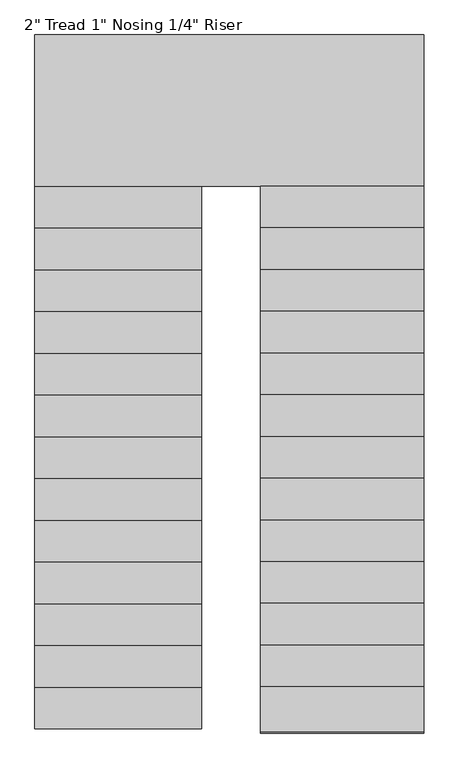
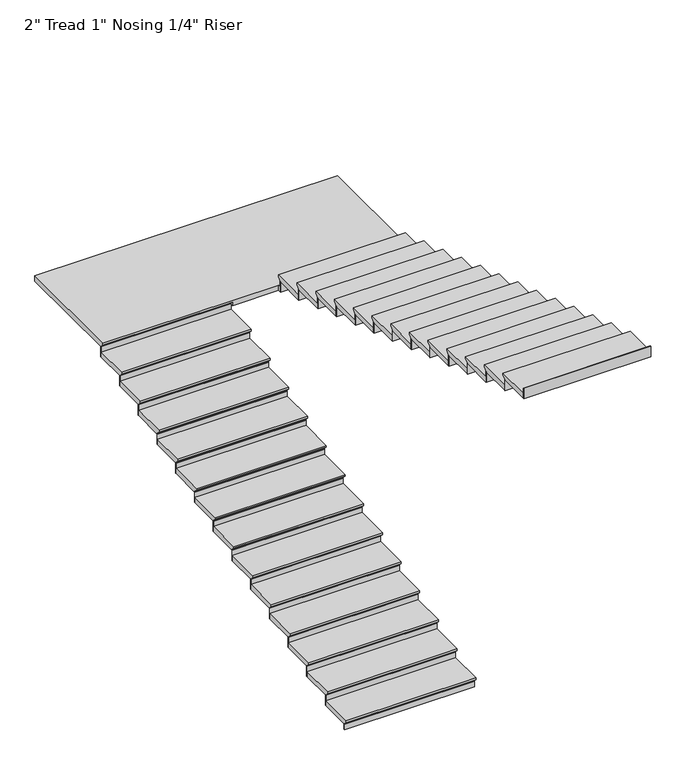
"""IFC4 building model written with IfcOpenShell, lengths in millimetres: stair flight geometry."""

from ifc_helpers import new_model, si_unit, origin, place, context, project, spatial, faceted_brep, source, transform, mapped, element, save


def stair_flight_d8047cd6(model_context):
    return source(origin(), model_context, "Body", "Brep", [
        faceted_brep([(-629.5987998, 2564.5067329, 16086.3642857), (-629.5987998, 2564.5067329, 16105.4142857), (-1848.7987998, 2564.5067329, 16105.4142857), (-1848.7987998, 2564.5067329, 16086.3642857), (-629.5987998, 2589.9067329, 16060.9642857), (-1848.7987998, 2589.9067329, 16060.9642857), (-629.5987998, 2894.7067329, 16105.4142857), (-1848.7987998, 2894.7067329, 16105.4142857), (-1848.7987998, 2589.9067329, 16054.6142857), (-1848.7987998, 2894.7067329, 16054.6142857), (-629.5987998, 2894.7067329, 16054.6142857), (-629.5987998, 2589.9067329, 16054.6142857)], [[[0, 1, 2, 3]], [[4, 0, 3, 5]], [[2, 1, 6, 7]], [[8, 9, 10, 11]], [[2, 7, 9, 8, 5, 3]], [[8, 11, 4, 5]], [[6, 1, 0, 4, 11, 10]], [[7, 6, 10, 9]]]),
        faceted_brep([(-629.5987998, 2589.9067329, 16054.6142857), (-629.5987998, 2589.9067329, 16002.0), (-629.5987998, 2596.2567329, 16002.0), (-629.5987998, 2596.2567329, 16054.6142857), (-1848.7987998, 2589.9067329, 16054.6142857), (-1848.7987998, 2596.2567329, 16054.6142857), (-1848.7987998, 2596.2567329, 16002.0), (-1848.7987998, 2589.9067329, 16002.0)], [[[0, 1, 2, 3]], [[4, 5, 6, 7]], [[1, 0, 4, 7]], [[2, 1, 7, 6]], [[3, 2, 6, 5]], [[0, 3, 5, 4]]]),
        faceted_brep([(-629.5987998, 2894.7067329, 16158.0285714), (-629.5987998, 2894.7067329, 16054.6142857), (-629.5987998, 2901.0567329, 16054.6142857), (-629.5987998, 2901.0567329, 16158.0285714), (-1848.7987998, 2894.7067329, 16158.0285714), (-1848.7987998, 2901.0567329, 16158.0285714), (-1848.7987998, 2901.0567329, 16054.6142857), (-1848.7987998, 2894.7067329, 16054.6142857)], [[[0, 1, 2, 3]], [[4, 5, 6, 7]], [[1, 0, 4, 7]], [[2, 1, 7, 6]], [[3, 2, 6, 5]], [[0, 3, 5, 4]]]),
        faceted_brep([(-1848.7987998, 2869.3067329, 16208.8285714), (-629.5987998, 2869.3067329, 16208.8285714), (-629.5987998, 3199.5067329, 16208.8285714), (-1848.7987998, 3199.5067329, 16208.8285714), (-1848.7987998, 2894.7067329, 16158.0285714), (-1848.7987998, 3199.5067329, 16158.0285714), (-629.5987998, 3199.5067329, 16158.0285714), (-629.5987998, 2894.7067329, 16158.0285714), (-1848.7987998, 2894.7067329, 16164.3785714), (-1848.7987998, 2869.3067329, 16189.7785714), (-629.5987998, 2894.7067329, 16164.3785714), (-629.5987998, 2869.3067329, 16189.7785714)], [[[0, 1, 2, 3]], [[4, 5, 6, 7]], [[0, 3, 5, 4, 8, 9]], [[4, 7, 10, 8]], [[2, 1, 11, 10, 7, 6]], [[3, 2, 6, 5]], [[11, 1, 0, 9]], [[10, 11, 9, 8]]]),
        faceted_brep([(-629.5987998, 3199.5067329, 16261.4428571), (-629.5987998, 3199.5067329, 16158.0285714), (-629.5987998, 3205.8567329, 16158.0285714), (-629.5987998, 3205.8567329, 16261.4428571), (-1848.7987998, 3199.5067329, 16261.4428571), (-1848.7987998, 3205.8567329, 16261.4428571), (-1848.7987998, 3205.8567329, 16158.0285714), (-1848.7987998, 3199.5067329, 16158.0285714)], [[[0, 1, 2, 3]], [[4, 5, 6, 7]], [[1, 0, 4, 7]], [[2, 1, 7, 6]], [[3, 2, 6, 5]], [[0, 3, 5, 4]]]),
        faceted_brep([(-1848.7987998, 3174.1067329, 16312.2428571), (-629.5987998, 3174.1067329, 16312.2428571), (-629.5987998, 3504.3067329, 16312.2428571), (-1848.7987998, 3504.3067329, 16312.2428571), (-1848.7987998, 3199.5067329, 16261.4428571), (-1848.7987998, 3504.3067329, 16261.4428571), (-629.5987998, 3504.3067329, 16261.4428571), (-629.5987998, 3199.5067329, 16261.4428571), (-1848.7987998, 3199.5067329, 16267.7928571), (-1848.7987998, 3174.1067329, 16293.1928571), (-629.5987998, 3199.5067329, 16267.7928571), (-629.5987998, 3174.1067329, 16293.1928571)], [[[0, 1, 2, 3]], [[4, 5, 6, 7]], [[0, 3, 5, 4, 8, 9]], [[4, 7, 10, 8]], [[2, 1, 11, 10, 7, 6]], [[3, 2, 6, 5]], [[11, 1, 0, 9]], [[10, 11, 9, 8]]]),
        faceted_brep([(-629.5987998, 3504.3067329, 16364.8571429), (-629.5987998, 3504.3067329, 16261.4428571), (-629.5987998, 3510.6567329, 16261.4428571), (-629.5987998, 3510.6567329, 16364.8571429), (-1848.7987998, 3504.3067329, 16364.8571429), (-1848.7987998, 3510.6567329, 16364.8571429), (-1848.7987998, 3510.6567329, 16261.4428571), (-1848.7987998, 3504.3067329, 16261.4428571)], [[[0, 1, 2, 3]], [[4, 5, 6, 7]], [[1, 0, 4, 7]], [[2, 1, 7, 6]], [[3, 2, 6, 5]], [[0, 3, 5, 4]]]),
        faceted_brep([(-1848.7987998, 3478.9067329, 16415.6571429), (-629.5987998, 3478.9067329, 16415.6571429), (-629.5987998, 3809.1067329, 16415.6571429), (-1848.7987998, 3809.1067329, 16415.6571429), (-1848.7987998, 3504.3067329, 16364.8571429), (-1848.7987998, 3809.1067329, 16364.8571429), (-629.5987998, 3809.1067329, 16364.8571429), (-629.5987998, 3504.3067329, 16364.8571429), (-1848.7987998, 3504.3067329, 16371.2071429), (-1848.7987998, 3478.9067329, 16396.6071429), (-629.5987998, 3504.3067329, 16371.2071429), (-629.5987998, 3478.9067329, 16396.6071429)], [[[0, 1, 2, 3]], [[4, 5, 6, 7]], [[0, 3, 5, 4, 8, 9]], [[4, 7, 10, 8]], [[2, 1, 11, 10, 7, 6]], [[3, 2, 6, 5]], [[11, 1, 0, 9]], [[10, 11, 9, 8]]]),
        faceted_brep([(-629.5987998, 3809.1067329, 16468.2714286), (-629.5987998, 3809.1067329, 16364.8571429), (-629.5987998, 3815.4567329, 16364.8571429), (-629.5987998, 3815.4567329, 16468.2714286), (-1848.7987998, 3809.1067329, 16468.2714286), (-1848.7987998, 3815.4567329, 16468.2714286), (-1848.7987998, 3815.4567329, 16364.8571429), (-1848.7987998, 3809.1067329, 16364.8571429)], [[[0, 1, 2, 3]], [[4, 5, 6, 7]], [[1, 0, 4, 7]], [[2, 1, 7, 6]], [[3, 2, 6, 5]], [[0, 3, 5, 4]]]),
        faceted_brep([(-1848.7987998, 3783.7067329, 16519.0714286), (-629.5987998, 3783.7067329, 16519.0714286), (-629.5987998, 4113.9067329, 16519.0714286), (-1848.7987998, 4113.9067329, 16519.0714286), (-1848.7987998, 3809.1067329, 16468.2714286), (-1848.7987998, 4113.9067329, 16468.2714286), (-629.5987998, 4113.9067329, 16468.2714286), (-629.5987998, 3809.1067329, 16468.2714286), (-1848.7987998, 3809.1067329, 16474.6214286), (-1848.7987998, 3783.7067329, 16500.0214286), (-629.5987998, 3809.1067329, 16474.6214286), (-629.5987998, 3783.7067329, 16500.0214286)], [[[0, 1, 2, 3]], [[4, 5, 6, 7]], [[0, 3, 5, 4, 8, 9]], [[4, 7, 10, 8]], [[2, 1, 11, 10, 7, 6]], [[3, 2, 6, 5]], [[11, 1, 0, 9]], [[10, 11, 9, 8]]]),
        faceted_brep([(-629.5987998, 4113.9067329, 16571.6857143), (-629.5987998, 4113.9067329, 16468.2714286), (-629.5987998, 4120.2567329, 16468.2714286), (-629.5987998, 4120.2567329, 16571.6857143), (-1848.7987998, 4113.9067329, 16571.6857143), (-1848.7987998, 4120.2567329, 16571.6857143), (-1848.7987998, 4120.2567329, 16468.2714286), (-1848.7987998, 4113.9067329, 16468.2714286)], [[[0, 1, 2, 3]], [[4, 5, 6, 7]], [[1, 0, 4, 7]], [[2, 1, 7, 6]], [[3, 2, 6, 5]], [[0, 3, 5, 4]]]),
        faceted_brep([(-1848.7987998, 4088.5067329, 16622.4857143), (-629.5987998, 4088.5067329, 16622.4857143), (-629.5987998, 4418.7067329, 16622.4857143), (-1848.7987998, 4418.7067329, 16622.4857143), (-1848.7987998, 4113.9067329, 16571.6857143), (-1848.7987998, 4418.7067329, 16571.6857143), (-629.5987998, 4418.7067329, 16571.6857143), (-629.5987998, 4113.9067329, 16571.6857143), (-1848.7987998, 4113.9067329, 16578.0357143), (-1848.7987998, 4088.5067329, 16603.4357143), (-629.5987998, 4113.9067329, 16578.0357143), (-629.5987998, 4088.5067329, 16603.4357143)], [[[0, 1, 2, 3]], [[4, 5, 6, 7]], [[0, 3, 5, 4, 8, 9]], [[4, 7, 10, 8]], [[2, 1, 11, 10, 7, 6]], [[3, 2, 6, 5]], [[11, 1, 0, 9]], [[10, 11, 9, 8]]]),
        faceted_brep([(-629.5987998, 4418.7067329, 16675.1), (-629.5987998, 4418.7067329, 16571.6857143), (-629.5987998, 4425.0567329, 16571.6857143), (-629.5987998, 4425.0567329, 16675.1), (-1848.7987998, 4418.7067329, 16675.1), (-1848.7987998, 4425.0567329, 16675.1), (-1848.7987998, 4425.0567329, 16571.6857143), (-1848.7987998, 4418.7067329, 16571.6857143)], [[[0, 1, 2, 3]], [[4, 5, 6, 7]], [[1, 0, 4, 7]], [[2, 1, 7, 6]], [[3, 2, 6, 5]], [[0, 3, 5, 4]]]),
        faceted_brep([(-1848.7987998, 4393.3067329, 16725.9), (-629.5987998, 4393.3067329, 16725.9), (-629.5987998, 4723.5067329, 16725.9), (-1848.7987998, 4723.5067329, 16725.9), (-1848.7987998, 4418.7067329, 16675.1), (-1848.7987998, 4723.5067329, 16675.1), (-629.5987998, 4723.5067329, 16675.1), (-629.5987998, 4418.7067329, 16675.1), (-1848.7987998, 4418.7067329, 16681.45), (-1848.7987998, 4393.3067329, 16706.85), (-629.5987998, 4418.7067329, 16681.45), (-629.5987998, 4393.3067329, 16706.85)], [[[0, 1, 2, 3]], [[4, 5, 6, 7]], [[0, 3, 5, 4, 8, 9]], [[4, 7, 10, 8]], [[2, 1, 11, 10, 7, 6]], [[3, 2, 6, 5]], [[11, 1, 0, 9]], [[10, 11, 9, 8]]]),
        faceted_brep([(-629.5987998, 4723.5067329, 16778.5142857), (-629.5987998, 4723.5067329, 16675.1), (-629.5987998, 4729.8567329, 16675.1), (-629.5987998, 4729.8567329, 16778.5142857), (-1848.7987998, 4723.5067329, 16778.5142857), (-1848.7987998, 4729.8567329, 16778.5142857), (-1848.7987998, 4729.8567329, 16675.1), (-1848.7987998, 4723.5067329, 16675.1)], [[[0, 1, 2, 3]], [[4, 5, 6, 7]], [[1, 0, 4, 7]], [[2, 1, 7, 6]], [[3, 2, 6, 5]], [[0, 3, 5, 4]]]),
        faceted_brep([(-1848.7987998, 4698.1067329, 16829.3142857), (-629.5987998, 4698.1067329, 16829.3142857), (-629.5987998, 5028.3067329, 16829.3142857), (-1848.7987998, 5028.3067329, 16829.3142857), (-1848.7987998, 4723.5067329, 16778.5142857), (-1848.7987998, 5028.3067329, 16778.5142857), (-629.5987998, 5028.3067329, 16778.5142857), (-629.5987998, 4723.5067329, 16778.5142857), (-1848.7987998, 4723.5067329, 16784.8642857), (-1848.7987998, 4698.1067329, 16810.2642857), (-629.5987998, 4723.5067329, 16784.8642857), (-629.5987998, 4698.1067329, 16810.2642857)], [[[0, 1, 2, 3]], [[4, 5, 6, 7]], [[0, 3, 5, 4, 8, 9]], [[4, 7, 10, 8]], [[2, 1, 11, 10, 7, 6]], [[3, 2, 6, 5]], [[11, 1, 0, 9]], [[10, 11, 9, 8]]]),
        faceted_brep([(-629.5987998, 5028.3067329, 16881.9285714), (-629.5987998, 5028.3067329, 16778.5142857), (-629.5987998, 5034.6567329, 16778.5142857), (-629.5987998, 5034.6567329, 16881.9285714), (-1848.7987998, 5028.3067329, 16881.9285714), (-1848.7987998, 5034.6567329, 16881.9285714), (-1848.7987998, 5034.6567329, 16778.5142857), (-1848.7987998, 5028.3067329, 16778.5142857)], [[[0, 1, 2, 3]], [[4, 5, 6, 7]], [[1, 0, 4, 7]], [[2, 1, 7, 6]], [[3, 2, 6, 5]], [[0, 3, 5, 4]]]),
        faceted_brep([(-1848.7987998, 5002.9067329, 16932.7285714), (-629.5987998, 5002.9067329, 16932.7285714), (-629.5987998, 5333.1067329, 16932.7285714), (-1848.7987998, 5333.1067329, 16932.7285714), (-1848.7987998, 5028.3067329, 16881.9285714), (-1848.7987998, 5333.1067329, 16881.9285714), (-629.5987998, 5333.1067329, 16881.9285714), (-629.5987998, 5028.3067329, 16881.9285714), (-1848.7987998, 5028.3067329, 16888.2785714), (-1848.7987998, 5002.9067329, 16913.6785714), (-629.5987998, 5028.3067329, 16888.2785714), (-629.5987998, 5002.9067329, 16913.6785714)], [[[0, 1, 2, 3]], [[4, 5, 6, 7]], [[0, 3, 5, 4, 8, 9]], [[4, 7, 10, 8]], [[2, 1, 11, 10, 7, 6]], [[3, 2, 6, 5]], [[11, 1, 0, 9]], [[10, 11, 9, 8]]]),
        faceted_brep([(-629.5987998, 5333.1067329, 16985.3428571), (-629.5987998, 5333.1067329, 16881.9285714), (-629.5987998, 5339.4567329, 16881.9285714), (-629.5987998, 5339.4567329, 16985.3428571), (-1848.7987998, 5333.1067329, 16985.3428571), (-1848.7987998, 5339.4567329, 16985.3428571), (-1848.7987998, 5339.4567329, 16881.9285714), (-1848.7987998, 5333.1067329, 16881.9285714)], [[[0, 1, 2, 3]], [[4, 5, 6, 7]], [[1, 0, 4, 7]], [[2, 1, 7, 6]], [[3, 2, 6, 5]], [[0, 3, 5, 4]]]),
        faceted_brep([(-1848.7987998, 5307.7067329, 17036.1428571), (-629.5987998, 5307.7067329, 17036.1428571), (-629.5987998, 5637.9067329, 17036.1428571), (-1848.7987998, 5637.9067329, 17036.1428571), (-1848.7987998, 5333.1067329, 16985.3428571), (-1848.7987998, 5637.9067329, 16985.3428571), (-629.5987998, 5637.9067329, 16985.3428571), (-629.5987998, 5333.1067329, 16985.3428571), (-1848.7987998, 5333.1067329, 16991.6928571), (-1848.7987998, 5307.7067329, 17017.0928571), (-629.5987998, 5333.1067329, 16991.6928571), (-629.5987998, 5307.7067329, 17017.0928571)], [[[0, 1, 2, 3]], [[4, 5, 6, 7]], [[0, 3, 5, 4, 8, 9]], [[4, 7, 10, 8]], [[2, 1, 11, 10, 7, 6]], [[3, 2, 6, 5]], [[11, 1, 0, 9]], [[10, 11, 9, 8]]]),
        faceted_brep([(-629.5987998, 5637.9067329, 17088.7571429), (-629.5987998, 5637.9067329, 16985.3428571), (-629.5987998, 5644.2567329, 16985.3428571), (-629.5987998, 5644.2567329, 17088.7571429), (-1848.7987998, 5637.9067329, 17088.7571429), (-1848.7987998, 5644.2567329, 17088.7571429), (-1848.7987998, 5644.2567329, 16985.3428571), (-1848.7987998, 5637.9067329, 16985.3428571)], [[[0, 1, 2, 3]], [[4, 5, 6, 7]], [[1, 0, 4, 7]], [[2, 1, 7, 6]], [[3, 2, 6, 5]], [[0, 3, 5, 4]]]),
        faceted_brep([(-1848.7987998, 5612.5067329, 17139.5571429), (-629.5987998, 5612.5067329, 17139.5571429), (-629.5987998, 5942.7067329, 17139.5571429), (-1848.7987998, 5942.7067329, 17139.5571429), (-1848.7987998, 5637.9067329, 17088.7571429), (-1848.7987998, 5942.7067329, 17088.7571429), (-629.5987998, 5942.7067329, 17088.7571429), (-629.5987998, 5637.9067329, 17088.7571429), (-1848.7987998, 5637.9067329, 17095.1071429), (-1848.7987998, 5612.5067329, 17120.5071429), (-629.5987998, 5637.9067329, 17095.1071429), (-629.5987998, 5612.5067329, 17120.5071429)], [[[0, 1, 2, 3]], [[4, 5, 6, 7]], [[0, 3, 5, 4, 8, 9]], [[4, 7, 10, 8]], [[2, 1, 11, 10, 7, 6]], [[3, 2, 6, 5]], [[11, 1, 0, 9]], [[10, 11, 9, 8]]]),
        faceted_brep([(-629.5987998, 5942.7067329, 17192.1714286), (-629.5987998, 5942.7067329, 17088.7571429), (-629.5987998, 5949.0567329, 17088.7571429), (-629.5987998, 5949.0567329, 17192.1714286), (-1848.7987998, 5942.7067329, 17192.1714286), (-1848.7987998, 5949.0567329, 17192.1714286), (-1848.7987998, 5949.0567329, 17088.7571429), (-1848.7987998, 5942.7067329, 17088.7571429)], [[[0, 1, 2, 3]], [[4, 5, 6, 7]], [[1, 0, 4, 7]], [[2, 1, 7, 6]], [[3, 2, 6, 5]], [[0, 3, 5, 4]]]),
        faceted_brep([(-1848.7987998, 5917.3067329, 17242.9714286), (-629.5987998, 5917.3067329, 17242.9714286), (-629.5987998, 6247.5067329, 17242.9714286), (-1848.7987998, 6247.5067329, 17242.9714286), (-1848.7987998, 5942.7067329, 17192.1714286), (-1848.7987998, 6247.5067329, 17192.1714286), (-629.5987998, 6247.5067329, 17192.1714286), (-629.5987998, 5942.7067329, 17192.1714286), (-1848.7987998, 5942.7067329, 17198.5214286), (-1848.7987998, 5917.3067329, 17223.9214286), (-629.5987998, 5942.7067329, 17198.5214286), (-629.5987998, 5917.3067329, 17223.9214286)], [[[0, 1, 2, 3]], [[4, 5, 6, 7]], [[0, 3, 5, 4, 8, 9]], [[4, 7, 10, 8]], [[2, 1, 11, 10, 7, 6]], [[3, 2, 6, 5]], [[11, 1, 0, 9]], [[10, 11, 9, 8]]]),
        faceted_brep([(-629.5987998, 6247.5067329, 17295.5857143), (-629.5987998, 6247.5067329, 17192.1714286), (-629.5987998, 6253.8567329, 17192.1714286), (-629.5987998, 6253.8567329, 17295.5857143), (-1848.7987998, 6247.5067329, 17295.5857143), (-1848.7987998, 6253.8567329, 17295.5857143), (-1848.7987998, 6253.8567329, 17192.1714286), (-1848.7987998, 6247.5067329, 17192.1714286)], [[[0, 1, 2, 3]], [[4, 5, 6, 7]], [[1, 0, 4, 7]], [[2, 1, 7, 6]], [[3, 2, 6, 5]], [[0, 3, 5, 4]]]),
        faceted_brep([(-1848.7987998, 6222.1067329, 17346.3857143), (-629.5987998, 6222.1067329, 17346.3857143), (-629.5987998, 6552.3067329, 17346.3857143), (-1848.7987998, 6552.3067329, 17346.3857143), (-1848.7987998, 6247.5067329, 17295.5857143), (-1848.7987998, 6552.3067329, 17295.5857143), (-629.5987998, 6552.3067329, 17295.5857143), (-629.5987998, 6247.5067329, 17295.5857143), (-1848.7987998, 6247.5067329, 17301.9357143), (-1848.7987998, 6222.1067329, 17327.3357143), (-629.5987998, 6247.5067329, 17301.9357143), (-629.5987998, 6222.1067329, 17327.3357143)], [[[0, 1, 2, 3]], [[4, 5, 6, 7]], [[0, 3, 5, 4, 8, 9]], [[4, 7, 10, 8]], [[2, 1, 11, 10, 7, 6]], [[3, 2, 6, 5]], [[11, 1, 0, 9]], [[10, 11, 9, 8]]]),
        faceted_brep([(-629.5987998, 6552.3067329, 17399.0), (-629.5987998, 6552.3067329, 17295.5857143), (-629.5987998, 6558.6567329, 17295.5857143), (-629.5987998, 6558.6567329, 17399.0), (-1848.7987998, 6552.3067329, 17399.0), (-1848.7987998, 6558.6567329, 17399.0), (-1848.7987998, 6558.6567329, 17295.5857143), (-1848.7987998, 6552.3067329, 17295.5857143)], [[[0, 1, 2, 3]], [[4, 5, 6, 7]], [[1, 0, 4, 7]], [[2, 1, 7, 6]], [[3, 2, 6, 5]], [[0, 3, 5, 4]]]),
        faceted_brep([(996.0012002, 6501.5067329, 17449.8), (996.0012002, 7631.8067329, 17449.8), (-1848.7987998, 7631.8067329, 17449.8), (-1848.7987998, 6526.9067329, 17449.8), (-197.7987915, 6526.9067329, 17449.8), (-197.7987915, 6501.5067329, 17449.8), (996.0012002, 7631.8067329, 17399.0), (996.0012002, 6501.5067329, 17399.0), (-197.7987915, 6501.5067329, 17399.0), (-197.7987915, 6526.9067329, 17399.0), (-629.5987998, 6526.9067329, 17399.0), (-629.5987998, 6552.3067329, 17399.0), (-1848.7987998, 6552.3067329, 17399.0), (-1848.7987998, 7631.8067329, 17399.0), (-629.5987998, 6552.3067329, 17405.35), (-1848.7987998, 6552.3067329, 17405.35), (-1848.7987998, 6526.9067329, 17430.75), (-629.5987998, 6526.9067329, 17430.75)], [[[0, 1, 2, 3, 4, 5]], [[6, 7, 8, 9, 10, 11, 12, 13]], [[1, 0, 7, 6]], [[2, 1, 6, 13]], [[12, 11, 14, 15]], [[4, 3, 16, 17, 10, 9]], [[5, 4, 9, 8]], [[0, 5, 8, 7]], [[16, 15, 14, 17]], [[3, 2, 13, 12, 15, 16]], [[11, 10, 17, 14]]]),
        faceted_brep([(-197.7987915, 6501.5067329, 17502.4142857), (-197.7987915, 6501.5067329, 17399.0), (-197.7987915, 6495.1567329, 17399.0), (-197.7987915, 6495.1567329, 17502.4142857), (996.0012002, 6501.5067329, 17502.4142857), (996.0012002, 6495.1567329, 17502.4142857), (996.0012002, 6495.1567329, 17399.0), (996.0012002, 6501.5067329, 17399.0)], [[[0, 1, 2, 3]], [[4, 5, 6, 7]], [[1, 0, 4, 7]], [[2, 1, 7, 6]], [[3, 2, 6, 5]], [[0, 3, 5, 4]]]),
        faceted_brep([(996.0012002, 6526.9067329, 17553.2142857), (-197.7987915, 6526.9067329, 17553.2142857), (-197.7987915, 6196.7067329, 17553.2142857), (996.0012002, 6196.7067329, 17553.2142857), (996.0012002, 6501.5067329, 17502.4142857), (996.0012002, 6196.7067329, 17502.4142857), (-197.7987915, 6196.7067329, 17502.4142857), (-197.7987915, 6501.5067329, 17502.4142857), (996.0012002, 6501.5067329, 17508.7642857), (996.0012002, 6526.9067329, 17534.1642857), (-197.7987915, 6501.5067329, 17508.7642857), (-197.7987915, 6526.9067329, 17534.1642857)], [[[0, 1, 2, 3]], [[4, 5, 6, 7]], [[0, 3, 5, 4, 8, 9]], [[4, 7, 10, 8]], [[2, 1, 11, 10, 7, 6]], [[3, 2, 6, 5]], [[11, 1, 0, 9]], [[10, 11, 9, 8]]]),
        faceted_brep([(-197.7987915, 6196.7067329, 17605.8285714), (-197.7987915, 6196.7067329, 17502.4142857), (-197.7987915, 6190.3567329, 17502.4142857), (-197.7987915, 6190.3567329, 17605.8285714), (996.0012002, 6196.7067329, 17605.8285714), (996.0012002, 6190.3567329, 17605.8285714), (996.0012002, 6190.3567329, 17502.4142857), (996.0012002, 6196.7067329, 17502.4142857)], [[[0, 1, 2, 3]], [[4, 5, 6, 7]], [[1, 0, 4, 7]], [[2, 1, 7, 6]], [[3, 2, 6, 5]], [[0, 3, 5, 4]]]),
        faceted_brep([(996.0012002, 6222.1067329, 17656.6285714), (-197.7987915, 6222.1067329, 17656.6285714), (-197.7987915, 5891.9067329, 17656.6285714), (996.0012002, 5891.9067329, 17656.6285714), (996.0012002, 6196.7067329, 17605.8285714), (996.0012002, 5891.9067329, 17605.8285714), (-197.7987915, 5891.9067329, 17605.8285714), (-197.7987915, 6196.7067329, 17605.8285714), (996.0012002, 6196.7067329, 17612.1785714), (996.0012002, 6222.1067329, 17637.5785714), (-197.7987915, 6196.7067329, 17612.1785714), (-197.7987915, 6222.1067329, 17637.5785714)], [[[0, 1, 2, 3]], [[4, 5, 6, 7]], [[0, 3, 5, 4, 8, 9]], [[4, 7, 10, 8]], [[2, 1, 11, 10, 7, 6]], [[3, 2, 6, 5]], [[11, 1, 0, 9]], [[10, 11, 9, 8]]]),
        faceted_brep([(-197.7987915, 5891.9067329, 17709.2428571), (-197.7987915, 5891.9067329, 17605.8285714), (-197.7987915, 5885.5567329, 17605.8285714), (-197.7987915, 5885.5567329, 17709.2428571), (996.0012002, 5891.9067329, 17709.2428571), (996.0012002, 5885.5567329, 17709.2428571), (996.0012002, 5885.5567329, 17605.8285714), (996.0012002, 5891.9067329, 17605.8285714)], [[[0, 1, 2, 3]], [[4, 5, 6, 7]], [[1, 0, 4, 7]], [[2, 1, 7, 6]], [[3, 2, 6, 5]], [[0, 3, 5, 4]]]),
        faceted_brep([(996.0012002, 5917.3067329, 17760.0428571), (-197.7987915, 5917.3067329, 17760.0428571), (-197.7987915, 5587.1067329, 17760.0428571), (996.0012002, 5587.1067329, 17760.0428571), (996.0012002, 5891.9067329, 17709.2428571), (996.0012002, 5587.1067329, 17709.2428571), (-197.7987915, 5587.1067329, 17709.2428571), (-197.7987915, 5891.9067329, 17709.2428571), (996.0012002, 5891.9067329, 17715.5928571), (996.0012002, 5917.3067329, 17740.9928571), (-197.7987915, 5891.9067329, 17715.5928571), (-197.7987915, 5917.3067329, 17740.9928571)], [[[0, 1, 2, 3]], [[4, 5, 6, 7]], [[0, 3, 5, 4, 8, 9]], [[4, 7, 10, 8]], [[2, 1, 11, 10, 7, 6]], [[3, 2, 6, 5]], [[11, 1, 0, 9]], [[10, 11, 9, 8]]]),
        faceted_brep([(-197.7987915, 5587.1067329, 17812.6571429), (-197.7987915, 5587.1067329, 17709.2428571), (-197.7987915, 5580.7567329, 17709.2428571), (-197.7987915, 5580.7567329, 17812.6571429), (996.0012002, 5587.1067329, 17812.6571429), (996.0012002, 5580.7567329, 17812.6571429), (996.0012002, 5580.7567329, 17709.2428571), (996.0012002, 5587.1067329, 17709.2428571)], [[[0, 1, 2, 3]], [[4, 5, 6, 7]], [[1, 0, 4, 7]], [[2, 1, 7, 6]], [[3, 2, 6, 5]], [[0, 3, 5, 4]]]),
        faceted_brep([(996.0012002, 5612.5067329, 17863.4571429), (-197.7987915, 5612.5067329, 17863.4571429), (-197.7987915, 5282.3067329, 17863.4571429), (996.0012002, 5282.3067329, 17863.4571429), (996.0012002, 5587.1067329, 17812.6571429), (996.0012002, 5282.3067329, 17812.6571429), (-197.7987915, 5282.3067329, 17812.6571429), (-197.7987915, 5587.1067329, 17812.6571429), (996.0012002, 5587.1067329, 17819.0071429), (996.0012002, 5612.5067329, 17844.4071429), (-197.7987915, 5587.1067329, 17819.0071429), (-197.7987915, 5612.5067329, 17844.4071429)], [[[0, 1, 2, 3]], [[4, 5, 6, 7]], [[0, 3, 5, 4, 8, 9]], [[4, 7, 10, 8]], [[2, 1, 11, 10, 7, 6]], [[3, 2, 6, 5]], [[11, 1, 0, 9]], [[10, 11, 9, 8]]]),
        faceted_brep([(-197.7987915, 5282.3067329, 17916.0714286), (-197.7987915, 5282.3067329, 17812.6571429), (-197.7987915, 5275.9567329, 17812.6571429), (-197.7987915, 5275.9567329, 17916.0714286), (996.0012002, 5282.3067329, 17916.0714286), (996.0012002, 5275.9567329, 17916.0714286), (996.0012002, 5275.9567329, 17812.6571429), (996.0012002, 5282.3067329, 17812.6571429)], [[[0, 1, 2, 3]], [[4, 5, 6, 7]], [[1, 0, 4, 7]], [[2, 1, 7, 6]], [[3, 2, 6, 5]], [[0, 3, 5, 4]]]),
        faceted_brep([(996.0012002, 5307.7067329, 17966.8714286), (-197.7987915, 5307.7067329, 17966.8714286), (-197.7987915, 4977.5067329, 17966.8714286), (996.0012002, 4977.5067329, 17966.8714286), (996.0012002, 5282.3067329, 17916.0714286), (996.0012002, 4977.5067329, 17916.0714286), (-197.7987915, 4977.5067329, 17916.0714286), (-197.7987915, 5282.3067329, 17916.0714286), (996.0012002, 5282.3067329, 17922.4214286), (996.0012002, 5307.7067329, 17947.8214286), (-197.7987915, 5282.3067329, 17922.4214286), (-197.7987915, 5307.7067329, 17947.8214286)], [[[0, 1, 2, 3]], [[4, 5, 6, 7]], [[0, 3, 5, 4, 8, 9]], [[4, 7, 10, 8]], [[2, 1, 11, 10, 7, 6]], [[3, 2, 6, 5]], [[11, 1, 0, 9]], [[10, 11, 9, 8]]]),
        faceted_brep([(-197.7987915, 4977.5067329, 18019.4857143), (-197.7987915, 4977.5067329, 17916.0714286), (-197.7987915, 4971.1567329, 17916.0714286), (-197.7987915, 4971.1567329, 18019.4857143), (996.0012002, 4977.5067329, 18019.4857143), (996.0012002, 4971.1567329, 18019.4857143), (996.0012002, 4971.1567329, 17916.0714286), (996.0012002, 4977.5067329, 17916.0714286)], [[[0, 1, 2, 3]], [[4, 5, 6, 7]], [[1, 0, 4, 7]], [[2, 1, 7, 6]], [[3, 2, 6, 5]], [[0, 3, 5, 4]]]),
        faceted_brep([(996.0012002, 5002.9067329, 18070.2857143), (-197.7987915, 5002.9067329, 18070.2857143), (-197.7987915, 4672.7067329, 18070.2857143), (996.0012002, 4672.7067329, 18070.2857143), (996.0012002, 4977.5067329, 18019.4857143), (996.0012002, 4672.7067329, 18019.4857143), (-197.7987915, 4672.7067329, 18019.4857143), (-197.7987915, 4977.5067329, 18019.4857143), (996.0012002, 4977.5067329, 18025.8357143), (996.0012002, 5002.9067329, 18051.2357143), (-197.7987915, 4977.5067329, 18025.8357143), (-197.7987915, 5002.9067329, 18051.2357143)], [[[0, 1, 2, 3]], [[4, 5, 6, 7]], [[0, 3, 5, 4, 8, 9]], [[4, 7, 10, 8]], [[2, 1, 11, 10, 7, 6]], [[3, 2, 6, 5]], [[11, 1, 0, 9]], [[10, 11, 9, 8]]]),
        faceted_brep([(-197.7987915, 4672.7067329, 18122.9), (-197.7987915, 4672.7067329, 18019.4857143), (-197.7987915, 4666.3567329, 18019.4857143), (-197.7987915, 4666.3567329, 18122.9), (996.0012002, 4672.7067329, 18122.9), (996.0012002, 4666.3567329, 18122.9), (996.0012002, 4666.3567329, 18019.4857143), (996.0012002, 4672.7067329, 18019.4857143)], [[[0, 1, 2, 3]], [[4, 5, 6, 7]], [[1, 0, 4, 7]], [[2, 1, 7, 6]], [[3, 2, 6, 5]], [[0, 3, 5, 4]]]),
        faceted_brep([(996.0012002, 4698.1067329, 18173.7), (-197.7987915, 4698.1067329, 18173.7), (-197.7987915, 4367.9067329, 18173.7), (996.0012002, 4367.9067329, 18173.7), (996.0012002, 4672.7067329, 18122.9), (996.0012002, 4367.9067329, 18122.9), (-197.7987915, 4367.9067329, 18122.9), (-197.7987915, 4672.7067329, 18122.9), (996.0012002, 4672.7067329, 18129.25), (996.0012002, 4698.1067329, 18154.65), (-197.7987915, 4672.7067329, 18129.25), (-197.7987915, 4698.1067329, 18154.65)], [[[0, 1, 2, 3]], [[4, 5, 6, 7]], [[0, 3, 5, 4, 8, 9]], [[4, 7, 10, 8]], [[2, 1, 11, 10, 7, 6]], [[3, 2, 6, 5]], [[11, 1, 0, 9]], [[10, 11, 9, 8]]]),
        faceted_brep([(-197.7987915, 4367.9067329, 18226.3142857), (-197.7987915, 4367.9067329, 18122.9), (-197.7987915, 4361.5567329, 18122.9), (-197.7987915, 4361.5567329, 18226.3142857), (996.0012002, 4367.9067329, 18226.3142857), (996.0012002, 4361.5567329, 18226.3142857), (996.0012002, 4361.5567329, 18122.9), (996.0012002, 4367.9067329, 18122.9)], [[[0, 1, 2, 3]], [[4, 5, 6, 7]], [[1, 0, 4, 7]], [[2, 1, 7, 6]], [[3, 2, 6, 5]], [[0, 3, 5, 4]]]),
        faceted_brep([(996.0012002, 4393.3067329, 18277.1142857), (-197.7987915, 4393.3067329, 18277.1142857), (-197.7987915, 4063.1067329, 18277.1142857), (996.0012002, 4063.1067329, 18277.1142857), (996.0012002, 4367.9067329, 18226.3142857), (996.0012002, 4063.1067329, 18226.3142857), (-197.7987915, 4063.1067329, 18226.3142857), (-197.7987915, 4367.9067329, 18226.3142857), (996.0012002, 4367.9067329, 18232.6642857), (996.0012002, 4393.3067329, 18258.0642857), (-197.7987915, 4367.9067329, 18232.6642857), (-197.7987915, 4393.3067329, 18258.0642857)], [[[0, 1, 2, 3]], [[4, 5, 6, 7]], [[0, 3, 5, 4, 8, 9]], [[4, 7, 10, 8]], [[2, 1, 11, 10, 7, 6]], [[3, 2, 6, 5]], [[11, 1, 0, 9]], [[10, 11, 9, 8]]]),
        faceted_brep([(-197.7987915, 4063.1067329, 18329.7285714), (-197.7987915, 4063.1067329, 18226.3142857), (-197.7987915, 4056.7567329, 18226.3142857), (-197.7987915, 4056.7567329, 18329.7285714), (996.0012002, 4063.1067329, 18329.7285714), (996.0012002, 4056.7567329, 18329.7285714), (996.0012002, 4056.7567329, 18226.3142857), (996.0012002, 4063.1067329, 18226.3142857)], [[[0, 1, 2, 3]], [[4, 5, 6, 7]], [[1, 0, 4, 7]], [[2, 1, 7, 6]], [[3, 2, 6, 5]], [[0, 3, 5, 4]]]),
        faceted_brep([(996.0012002, 4088.5067329, 18380.5285714), (-197.7987915, 4088.5067329, 18380.5285714), (-197.7987915, 3758.3067329, 18380.5285714), (996.0012002, 3758.3067329, 18380.5285714), (996.0012002, 4063.1067329, 18329.7285714), (996.0012002, 3758.3067329, 18329.7285714), (-197.7987915, 3758.3067329, 18329.7285714), (-197.7987915, 4063.1067329, 18329.7285714), (996.0012002, 4063.1067329, 18336.0785714), (996.0012002, 4088.5067329, 18361.4785714), (-197.7987915, 4063.1067329, 18336.0785714), (-197.7987915, 4088.5067329, 18361.4785714)], [[[0, 1, 2, 3]], [[4, 5, 6, 7]], [[0, 3, 5, 4, 8, 9]], [[4, 7, 10, 8]], [[2, 1, 11, 10, 7, 6]], [[3, 2, 6, 5]], [[11, 1, 0, 9]], [[10, 11, 9, 8]]]),
        faceted_brep([(-197.7987915, 3758.3067329, 18433.1428571), (-197.7987915, 3758.3067329, 18329.7285714), (-197.7987915, 3751.9567329, 18329.7285714), (-197.7987915, 3751.9567329, 18433.1428571), (996.0012002, 3758.3067329, 18433.1428571), (996.0012002, 3751.9567329, 18433.1428571), (996.0012002, 3751.9567329, 18329.7285714), (996.0012002, 3758.3067329, 18329.7285714)], [[[0, 1, 2, 3]], [[4, 5, 6, 7]], [[1, 0, 4, 7]], [[2, 1, 7, 6]], [[3, 2, 6, 5]], [[0, 3, 5, 4]]]),
        faceted_brep([(996.0012002, 3783.7067329, 18483.9428571), (-197.7987915, 3783.7067329, 18483.9428571), (-197.7987915, 3453.5067329, 18483.9428571), (996.0012002, 3453.5067329, 18483.9428571), (996.0012002, 3758.3067329, 18433.1428571), (996.0012002, 3453.5067329, 18433.1428571), (-197.7987915, 3453.5067329, 18433.1428571), (-197.7987915, 3758.3067329, 18433.1428571), (996.0012002, 3758.3067329, 18439.4928571), (996.0012002, 3783.7067329, 18464.8928571), (-197.7987915, 3758.3067329, 18439.4928571), (-197.7987915, 3783.7067329, 18464.8928571)], [[[0, 1, 2, 3]], [[4, 5, 6, 7]], [[0, 3, 5, 4, 8, 9]], [[4, 7, 10, 8]], [[2, 1, 11, 10, 7, 6]], [[3, 2, 6, 5]], [[11, 1, 0, 9]], [[10, 11, 9, 8]]]),
        faceted_brep([(-197.7987915, 3453.5067329, 18536.5571429), (-197.7987915, 3453.5067329, 18433.1428571), (-197.7987915, 3447.1567329, 18433.1428571), (-197.7987915, 3447.1567329, 18536.5571429), (996.0012002, 3453.5067329, 18536.5571429), (996.0012002, 3447.1567329, 18536.5571429), (996.0012002, 3447.1567329, 18433.1428571), (996.0012002, 3453.5067329, 18433.1428571)], [[[0, 1, 2, 3]], [[4, 5, 6, 7]], [[1, 0, 4, 7]], [[2, 1, 7, 6]], [[3, 2, 6, 5]], [[0, 3, 5, 4]]]),
        faceted_brep([(996.0012002, 3478.9067329, 18587.3571429), (-197.7987915, 3478.9067329, 18587.3571429), (-197.7987915, 3148.7067329, 18587.3571429), (996.0012002, 3148.7067329, 18587.3571429), (996.0012002, 3453.5067329, 18536.5571429), (996.0012002, 3148.7067329, 18536.5571429), (-197.7987915, 3148.7067329, 18536.5571429), (-197.7987915, 3453.5067329, 18536.5571429), (996.0012002, 3453.5067329, 18542.9071429), (996.0012002, 3478.9067329, 18568.3071429), (-197.7987915, 3453.5067329, 18542.9071429), (-197.7987915, 3478.9067329, 18568.3071429)], [[[0, 1, 2, 3]], [[4, 5, 6, 7]], [[0, 3, 5, 4, 8, 9]], [[4, 7, 10, 8]], [[2, 1, 11, 10, 7, 6]], [[3, 2, 6, 5]], [[11, 1, 0, 9]], [[10, 11, 9, 8]]]),
        faceted_brep([(-197.7987915, 3148.7067329, 18639.9714286), (-197.7987915, 3148.7067329, 18536.5571429), (-197.7987915, 3142.3567329, 18536.5571429), (-197.7987915, 3142.3567329, 18639.9714286), (996.0012002, 3148.7067329, 18639.9714286), (996.0012002, 3142.3567329, 18639.9714286), (996.0012002, 3142.3567329, 18536.5571429), (996.0012002, 3148.7067329, 18536.5571429)], [[[0, 1, 2, 3]], [[4, 5, 6, 7]], [[1, 0, 4, 7]], [[2, 1, 7, 6]], [[3, 2, 6, 5]], [[0, 3, 5, 4]]]),
        faceted_brep([(996.0012002, 3174.1067329, 18690.7714286), (-197.7987915, 3174.1067329, 18690.7714286), (-197.7987915, 2843.9067329, 18690.7714286), (996.0012002, 2843.9067329, 18690.7714286), (996.0012002, 3148.7067329, 18639.9714286), (996.0012002, 2843.9067329, 18639.9714286), (-197.7987915, 2843.9067329, 18639.9714286), (-197.7987915, 3148.7067329, 18639.9714286), (996.0012002, 3148.7067329, 18646.3214286), (996.0012002, 3174.1067329, 18671.7214286), (-197.7987915, 3148.7067329, 18646.3214286), (-197.7987915, 3174.1067329, 18671.7214286)], [[[0, 1, 2, 3]], [[4, 5, 6, 7]], [[0, 3, 5, 4, 8, 9]], [[4, 7, 10, 8]], [[2, 1, 11, 10, 7, 6]], [[3, 2, 6, 5]], [[11, 1, 0, 9]], [[10, 11, 9, 8]]]),
        faceted_brep([(-197.7987915, 2843.9067329, 18743.3857143), (-197.7987915, 2843.9067329, 18639.9714286), (-197.7987915, 2837.5567329, 18639.9714286), (-197.7987915, 2837.5567329, 18743.3857143), (996.0012002, 2843.9067329, 18743.3857143), (996.0012002, 2837.5567329, 18743.3857143), (996.0012002, 2837.5567329, 18639.9714286), (996.0012002, 2843.9067329, 18639.9714286)], [[[0, 1, 2, 3]], [[4, 5, 6, 7]], [[1, 0, 4, 7]], [[2, 1, 7, 6]], [[3, 2, 6, 5]], [[0, 3, 5, 4]]]),
        faceted_brep([(-197.7987915, 2539.1067329, 18846.8), (-197.7987915, 2539.1067329, 18743.3857143), (-197.7987915, 2532.7567329, 18743.3857143), (-197.7987915, 2532.7567329, 18846.8), (996.0012002, 2539.1067329, 18846.8), (996.0012002, 2532.7567329, 18846.8), (996.0012002, 2532.7567329, 18743.3857143), (996.0012002, 2539.1067329, 18743.3857143)], [[[0, 1, 2, 3]], [[4, 5, 6, 7]], [[1, 0, 4, 7]], [[2, 1, 7, 6]], [[3, 2, 6, 5]], [[0, 3, 5, 4]]]),
        faceted_brep([(996.0012002, 2869.3067329, 18794.1857143), (-197.7987915, 2869.3067329, 18794.1857143), (-197.7987915, 2539.1067329, 18794.1857143), (996.0012002, 2539.1067329, 18794.1857143), (996.0012002, 2843.9067329, 18743.3857143), (996.0012002, 2539.1067329, 18743.3857143), (-197.7987915, 2539.1067329, 18743.3857143), (-197.7987915, 2843.9067329, 18743.3857143), (996.0012002, 2843.9067329, 18749.7357143), (996.0012002, 2869.3067329, 18775.1357143), (-197.7987915, 2843.9067329, 18749.7357143), (-197.7987915, 2869.3067329, 18775.1357143)], [[[0, 1, 2, 3]], [[4, 5, 6, 7]], [[0, 3, 5, 4, 8, 9]], [[4, 7, 10, 8]], [[2, 1, 11, 10, 7, 6]], [[3, 2, 6, 5]], [[11, 1, 0, 9]], [[10, 11, 9, 8]]]),
    ])


if __name__ == "__main__":
    model = new_model("IFC4")
    model_context = context("Model", 3, world=origin())
    ifc_project = project(units=[si_unit("LENGTHUNIT", "METRE", prefix="MILLI")], contexts=[model_context])
    site = spatial("IfcSite", under=ifc_project)
    building = spatial("IfcBuilding", under=site)
    placement = place(None, origin())
    stair_flight_shape = stair_flight_d8047cd6(model_context)
    element("IfcStairFlight", 1, ObjectType="2\" Tread 1\" Nosing 1/4\" Riser", at=placement, inside=building, context=model_context, shape_type="MappedRepresentation", body=[
        mapped(stair_flight_shape, transform((0.0, 0.0, 0.0), x_axis=(1.0, 0.0, 0.0), y_axis=(0.0, 1.0, 0.0), z_axis=(0.0, 0.0, 1.0))),
    ])
    save(model, "model.ifc")
